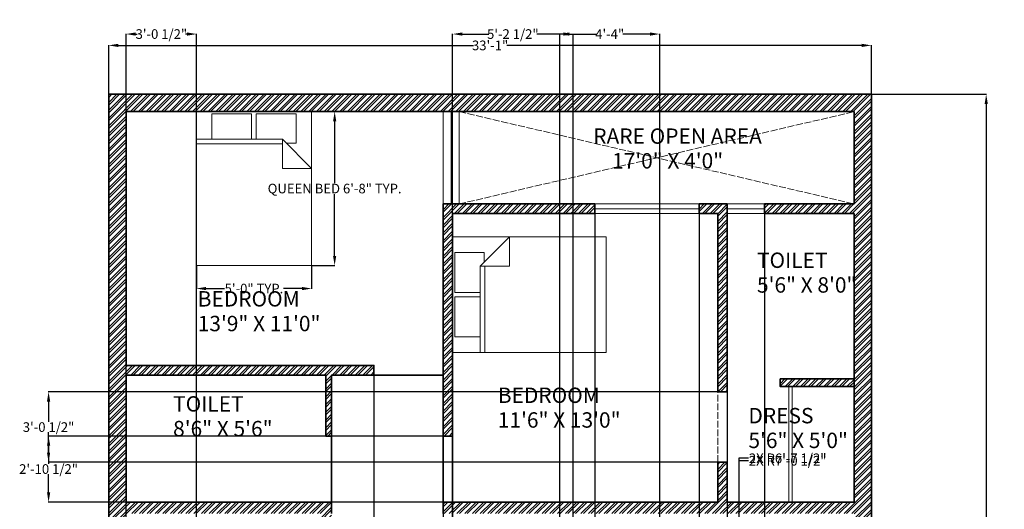
# Model space of a CAD drawing. Units: inches. Extents: x 334 to 846, y -424 to 250.
# Tile 3 of 3: x 334 to 846, y -5 to 250. Entities that reach past the tile are written whole.
import ezdxf

# ---------------------------------------------------------------- set-up
doc = ezdxf.new("R2010")
doc.units = ezdxf.units.IN
doc.header["$MEASUREMENT"] = 0
doc.linetypes.add('ACAD_ISO02W100', pattern=[15, 12, -3])
for name, color, linetype, lineweight in [('A-AREA-IDEN', 130, 'Continuous', 18), ('A-FLOR-FIXT', 8, 'Continuous', 18), ('A-FLOR-OPEN', 8, 'ACAD_ISO02W100', 13), ('A-WALL', 7, 'Continuous', 35), ('A-WALL-OVHD', 8, 'ACAD_ISO02W100', 18), ('A-WALL-PATT', 252, 'Continuous', 13), ('dimension', 130, 'Continuous', 18), ('furniture', 6, 'Continuous', 18), ('window', 150, 'Continuous', 18)]:
    doc.layers.add(name, color=color, linetype=linetype, lineweight=lineweight)
doc.styles.get("Standard").update_dxf_attribs({"font": 'arial.ttf'})
doc.dimstyles.get("Standard").update_dxf_attribs({"dimtxt": 5, "dimasz": 5, "dimexe": 0.18, "dimexo": 0.0625, "dimgap": 0.09, "dimtad": 0, "dimtih": 1, "dimtoh": 1, "dimdec": 1, "dimzin": 0, "dimdsep": 46, "dimlunit": 4, "dimtxsty": 'Standard', "dimcen": 0.09, "dimadec": 0, "dimazin": 0, "dimtfac": 1, "dimtdec": 1, "dimtofl": 0, "dimtmove": 0, "dimatfit": 3, "dimfxl": 1, "dimtolj": 1, "dimtzin": 0, "dimarcsym": 0})

# ---------------------------------------------------------------- blocks, each defined once
blk = doc.blocks.new('Bed - Queen')
for p, q in [((0, -80.00003), (0, 0)), ((0, 0), (59.99999, 0)), ((59.99999, 0), (59.99999, -80.00003)), ((7.99999, -1.2), (28.79998, -1.2)), ((7.99999, -14.4), (7.99999, -1.2)), ((28.79998, -1.2), (28.79998, -14.4)), ((31.19999, -1.2), (51.99999, -1.2)), ((31.19999, -14.4), (31.19999, -1.2)), ((51.99999, -1.2), (51.99999, -16.4)), ((0, -14.4), (44.8, -14.4)), ((59.99999, -29.6), (44.8, -14.4)), ((44.8, -14.4), (44.8, -29.6)), ((44.8, -16.8), (0, -16.8)), ((51.99999, -16.4), (46.79936, -16.4)), ((44.8, -29.6), (59.99999, -29.6)), ((59.99999, -80.00003), (0, -80.00003))]:
    blk.add_line(p, q)
blk = doc.blocks.new('*D7')
at = {"layer": 'Defpoints', "color": 0, "ltscale": 0.3, "transparency": 16777216}
for p in [(777.06, 236.45), (380.06, 211), (777.06, 211)]:
    blk.add_point(p, dxfattribs=at)
at = {"layer": 'dimension', "color": 0, "lineweight": -2, "ltscale": 0.3, "transparency": 16777216}
for p, q in [((380.06, 211.06), (380.06, 236.63)), ((385.06, 236.45), (569.89, 236.45)), ((772.06, 236.45), (587.24, 236.45)), ((777.06, 211.06), (777.06, 236.63))]:
    blk.add_line(p, q, dxfattribs=at)
at = {"layer": 'dimension', "color": 0, "ltscale": 0.3, "transparency": 16777216}
for points in [[(385.06, 237.28), (385.06, 235.61), (380.06, 236.45)], [(772.06, 237.28), (772.06, 235.61), (777.06, 236.45)]]:
    blk.add_solid(points, dxfattribs=at)
at = {"layer": 'dimension', "color": 0, "ltscale": 0.3, "transparency": 16777216, "insert": (578.56, 236.45), "char_height": 5, "attachment_point": 5}
blk.add_mtext('\\A1;33\'-1"', dxfattribs=at)
blk = doc.blocks.new('*D8')
at = {"layer": 'Defpoints', "color": 0, "ltscale": 0.3, "transparency": 16777216}
for p in [(777.06, 211), (777.06, -385), (836.82, -385)]:
    blk.add_point(p, dxfattribs=at)
at = {"layer": 'dimension', "color": 0, "lineweight": -2, "ltscale": 0.3, "transparency": 16777216}
for p, q in [((777.12, 211), (837, 211)), ((836.82, 206), (836.82, -84.36)), ((836.82, -380), (836.82, -89.65)), ((777.12, -385), (837, -385))]:
    blk.add_line(p, q, dxfattribs=at)
at = {"layer": 'dimension', "color": 0, "ltscale": 0.3, "transparency": 16777216}
for points in [[(835.99, 206), (837.66, 206), (836.82, 211)], [(835.99, -380), (837.66, -380), (836.82, -385)]]:
    blk.add_solid(points, dxfattribs=at)
at = {"layer": 'dimension', "color": 0, "ltscale": 0.3, "transparency": 16777216, "insert": (836.82, -87), "char_height": 5, "attachment_point": 5}
blk.add_mtext('\\A1;49\'-8"', dxfattribs=at)
blk = doc.blocks.new('*D10')
at = {"layer": 'Defpoints', "color": 0, "ltscale": 0.3, "transparency": 16777216}
for p in [(485.63, 202), (497.63, 202), (485.63, 122)]:
    blk.add_point(p, dxfattribs=at)
at = {"layer": 'dimension', "color": 0, "lineweight": -2, "ltscale": 0.3, "transparency": 16777216}
for p, q in [((485.69, 202), (497.81, 202)), ((497.63, 197), (497.63, 164.82)), ((497.63, 127), (497.63, 159.17)), ((485.69, 122), (497.81, 122))]:
    blk.add_line(p, q, dxfattribs=at)
at = {"layer": 'dimension', "color": 0, "ltscale": 0.3, "transparency": 16777216}
for points in [[(496.8, 197), (498.47, 197), (497.63, 202)], [(496.8, 127), (498.47, 127), (497.63, 122)]]:
    blk.add_solid(points, dxfattribs=at)
at = {"layer": 'dimension', "color": 0, "ltscale": 0.3, "transparency": 16777216, "insert": (497.63, 162), "char_height": 5, "attachment_point": 5}
blk.add_mtext('\\A1;QUEEN BED 6\'-8" TYP.', dxfattribs=at)
blk = doc.blocks.new('*D11')
at = {"layer": 'Defpoints', "color": 0, "ltscale": 0.3, "transparency": 16777216}
for p in [(425.63, 122), (485.63, 122), (485.63, 110)]:
    blk.add_point(p, dxfattribs=at)
at = {"layer": 'dimension', "color": 0, "lineweight": -2, "ltscale": 0.3, "transparency": 16777216}
for p, q in [((425.63, 121.93), (425.63, 109.82)), ((485.63, 121.93), (485.63, 109.82)), ((430.63, 110), (440.3, 110)), ((480.63, 110), (470.96, 110))]:
    blk.add_line(p, q, dxfattribs=at)
at = {"layer": 'dimension', "color": 0, "ltscale": 0.3, "transparency": 16777216}
for points in [[(430.63, 110.83), (430.63, 109.16), (425.63, 110)], [(480.63, 110.83), (480.63, 109.16), (485.63, 110)]]:
    blk.add_solid(points, dxfattribs=at)
at = {"layer": 'dimension', "color": 0, "ltscale": 0.3, "transparency": 16777216, "insert": (455.63, 110), "char_height": 5, "attachment_point": 5}
blk.add_mtext('\\A1;5\'-0" TYP.', dxfattribs=at)
blk = doc.blocks.new('*D20')
at = {"layer": 'Defpoints', "color": 0, "ltscale": 0.3, "transparency": 16777216}
for p in [(559.06, 149), (633.1, 149), (633.1, -416.35)]:
    blk.add_point(p, dxfattribs=at)
at = {"layer": 'dimension', "color": 0, "lineweight": -2, "ltscale": 0.3, "transparency": 16777216}
for p, q in [((559.06, 148.93), (559.06, -416.53)), ((633.1, 148.93), (633.1, -416.53)), ((564.06, -416.35), (589.33, -416.35)), ((628.1, -416.35), (602.83, -416.35))]:
    blk.add_line(p, q, dxfattribs=at)
at = {"layer": 'dimension', "color": 0, "ltscale": 0.3, "transparency": 16777216}
for points in [[(564.06, -415.52), (564.06, -417.19), (559.06, -416.35)], [(628.1, -415.52), (628.1, -417.19), (633.1, -416.35)]]:
    blk.add_solid(points, dxfattribs=at)
at = {"layer": 'dimension', "color": 0, "ltscale": 0.3, "transparency": 16777216, "insert": (596.08, -416.35), "char_height": 5, "attachment_point": 5}
blk.add_mtext('\\A1;6\'-2"', dxfattribs=at)
blk = doc.blocks.new('*D21')
at = {"layer": 'Defpoints', "color": 0, "ltscale": 0.3, "transparency": 16777216}
for p in [(633.1, 149), (687.41, 149), (687.41, -416.35)]:
    blk.add_point(p, dxfattribs=at)
at = {"layer": 'dimension', "color": 0, "lineweight": -2, "ltscale": 0.3, "transparency": 16777216}
for p, q in [((633.1, 148.93), (633.1, -416.53)), ((687.41, 148.93), (687.41, -416.53)), ((638.1, -416.35), (647.59, -416.35)), ((682.41, -416.35), (672.92, -416.35))]:
    blk.add_line(p, q, dxfattribs=at)
at = {"layer": 'dimension', "color": 0, "ltscale": 0.3, "transparency": 16777216}
for points in [[(638.1, -415.52), (638.1, -417.19), (633.1, -416.35)], [(682.41, -415.52), (682.41, -417.19), (687.41, -416.35)]]:
    blk.add_solid(points, dxfattribs=at)
at = {"layer": 'dimension', "color": 0, "ltscale": 0.3, "transparency": 16777216, "insert": (660.26, -416.35), "char_height": 5, "attachment_point": 5}
blk.add_mtext('\\A1;4\'-6 1/2"', dxfattribs=at)
blk = doc.blocks.new('*D22')
at = {"layer": 'Defpoints', "color": 0, "ltscale": 0.3, "transparency": 16777216}
for p in [(702.06, 149), (721.47, 149), (721.47, -416.35)]:
    blk.add_point(p, dxfattribs=at)
at = {"layer": 'dimension', "color": 0, "lineweight": -2, "ltscale": 0.3, "transparency": 16777216}
for p, q in [((702.06, 148.93), (702.06, -416.53)), ((721.47, 148.93), (721.47, -416.53)), ((707.06, -416.35), (716.47, -416.35)), ((721.47, -416.35), (726.47, -416.35))]:
    blk.add_line(p, q, dxfattribs=at)
at = {"layer": 'dimension', "color": 0, "ltscale": 0.3, "transparency": 16777216}
for points in [[(707.06, -415.52), (707.06, -417.19), (702.06, -416.35)], [(716.47, -415.52), (716.47, -417.19), (721.47, -416.35)]]:
    blk.add_solid(points, dxfattribs=at)
at = {"layer": 'dimension', "color": 0, "ltscale": 0.3, "transparency": 16777216, "insert": (738.8, -416.35), "char_height": 5, "attachment_point": 5}
blk.add_mtext('\\A1;1\'-7 1/2"', dxfattribs=at)
blk = doc.blocks.new('*D23')
at = {"layer": 'Defpoints', "color": 0, "ltscale": 0.3, "transparency": 16777216}
for p in [(518.06, 70), (554.06, 65), (554.06, -416.35)]:
    blk.add_point(p, dxfattribs=at)
at = {"layer": 'dimension', "color": 0, "lineweight": -2, "ltscale": 0.3, "transparency": 16777216}
for p, q in [((518.06, 69.93), (518.06, -416.53)), ((554.06, 64.93), (554.06, -416.53)), ((523.06, -416.35), (529.33, -416.35)), ((549.06, -416.35), (542.8, -416.35))]:
    blk.add_line(p, q, dxfattribs=at)
at = {"layer": 'dimension', "color": 0, "ltscale": 0.3, "transparency": 16777216}
for points in [[(523.06, -415.52), (523.06, -417.19), (518.06, -416.35)], [(549.06, -415.52), (549.06, -417.19), (554.06, -416.35)]]:
    blk.add_solid(points, dxfattribs=at)
at = {"layer": 'dimension', "color": 0, "ltscale": 0.3, "transparency": 16777216, "insert": (536.06, -416.35), "char_height": 5, "attachment_point": 5}
blk.add_mtext('\\A1;3\'-0"', dxfattribs=at)
blk = doc.blocks.new('*D24')
at = {"layer": 'Defpoints', "color": 0, "ltscale": 0.3, "transparency": 16777216}
for p in [(554.06, 33.31), (348.71, -1), (554.06, -1)]:
    blk.add_point(p, dxfattribs=at)
at = {"layer": 'dimension', "color": 0, "lineweight": -2, "ltscale": 0.3, "transparency": 16777216}
for p, q in [((554, 33.31), (348.53, 33.31)), ((348.71, 28.31), (348.71, 18.83)), ((348.71, 4), (348.71, 13.48)), ((554, -1), (348.53, -1))]:
    blk.add_line(p, q, dxfattribs=at)
at = {"layer": 'dimension', "color": 0, "ltscale": 0.3, "transparency": 16777216}
for points in [[(347.88, 28.31), (349.55, 28.31), (348.71, 33.31)], [(347.88, 4), (349.55, 4), (348.71, -1)]]:
    blk.add_solid(points, dxfattribs=at)
at = {"layer": 'dimension', "color": 0, "ltscale": 0.3, "transparency": 16777216, "insert": (348.71, 16.15), "char_height": 5, "attachment_point": 5}
blk.add_mtext('\\A1;2\'-10 1/2"', dxfattribs=at)
blk = doc.blocks.new('*D25')
at = {"layer": 'Defpoints', "color": 0, "ltscale": 0.3, "transparency": 16777216}
for p in [(496.06, 33.31), (348.71, -1), (496.06, -1)]:
    blk.add_point(p, dxfattribs=at)
at = {"layer": 'dimension', "color": 0, "lineweight": -2, "ltscale": 0.3, "transparency": 16777216}
for p, q in [((496, 33.31), (348.53, 33.31)), ((348.71, 28.31), (348.71, 18.83)), ((348.71, 4), (348.71, 13.48)), ((496, -1), (348.53, -1))]:
    blk.add_line(p, q, dxfattribs=at)
at = {"layer": 'dimension', "color": 0, "ltscale": 0.3, "transparency": 16777216}
for points in [[(347.88, 28.31), (349.55, 28.31), (348.71, 33.31)], [(347.88, 4), (349.55, 4), (348.71, -1)]]:
    blk.add_solid(points, dxfattribs=at)
at = {"layer": 'dimension', "color": 0, "ltscale": 0.3, "transparency": 16777216, "insert": (348.71, 16.15), "char_height": 5, "attachment_point": 5}
blk.add_mtext('\\A1;2\'-10 1/2"', dxfattribs=at)
blk = doc.blocks.new('*D26')
at = {"layer": 'Defpoints', "color": 0, "ltscale": 0.3, "transparency": 16777216}
for p in [(697.06, 56.25), (348.71, 19.69), (697.06, 19.69)]:
    blk.add_point(p, dxfattribs=at)
at = {"layer": 'dimension', "color": 0, "lineweight": -2, "ltscale": 0.3, "transparency": 16777216}
for p, q in [((697, 56.25), (348.53, 56.25)), ((348.71, 51.25), (348.71, 40.65)), ((348.71, 24.69), (348.71, 35.3)), ((697, 19.69), (348.53, 19.69))]:
    blk.add_line(p, q, dxfattribs=at)
at = {"layer": 'dimension', "color": 0, "ltscale": 0.3, "transparency": 16777216}
for points in [[(347.88, 51.25), (349.55, 51.25), (348.71, 56.25)], [(347.88, 24.69), (349.55, 24.69), (348.71, 19.69)]]:
    blk.add_solid(points, dxfattribs=at)
at = {"layer": 'dimension', "color": 0, "ltscale": 0.3, "transparency": 16777216, "insert": (348.71, 37.97), "char_height": 5, "attachment_point": 5}
blk.add_mtext('\\A1;3\'-0 1/2"', dxfattribs=at)
blk = doc.blocks.new('*D28')
at = {"layer": 'Defpoints', "color": 0, "ltscale": 0.3, "transparency": 16777216}
for p in [(666.86, 242.35), (614.79, -145), (666.86, -145)]:
    blk.add_point(p, dxfattribs=at)
at = {"layer": 'dimension', "color": 0, "lineweight": -2, "ltscale": 0.3, "transparency": 16777216}
for p, q in [((614.79, -144.94), (614.79, 242.53)), ((619.79, 242.35), (633.99, 242.35)), ((661.86, 242.35), (647.66, 242.35)), ((666.86, -144.94), (666.86, 242.53))]:
    blk.add_line(p, q, dxfattribs=at)
at = {"layer": 'dimension', "color": 0, "ltscale": 0.3, "transparency": 16777216}
for points in [[(619.79, 243.18), (619.79, 241.51), (614.79, 242.35)], [(661.86, 243.18), (661.86, 241.51), (666.86, 242.35)]]:
    blk.add_solid(points, dxfattribs=at)
at = {"layer": 'dimension', "color": 0, "ltscale": 0.3, "transparency": 16777216, "insert": (640.83, 242.35), "char_height": 5, "attachment_point": 5}
blk.add_mtext('\\A1;4\'-4"', dxfattribs=at)
blk = doc.blocks.new('*D30')
at = {"layer": 'Defpoints', "color": 0, "ltscale": 0.3, "transparency": 16777216}
for p in [(621.73, 242.35), (559.06, -271), (621.73, -271)]:
    blk.add_point(p, dxfattribs=at)
at = {"layer": 'dimension', "color": 0, "lineweight": -2, "ltscale": 0.3, "transparency": 16777216}
for p, q in [((559.06, -270.94), (559.06, 242.53)), ((564.06, 242.35), (577.83, 242.35)), ((616.73, 242.35), (602.96, 242.35)), ((621.73, -270.94), (621.73, 242.53))]:
    blk.add_line(p, q, dxfattribs=at)
at = {"layer": 'dimension', "color": 0, "ltscale": 0.3, "transparency": 16777216}
for points in [[(564.06, 243.18), (564.06, 241.51), (559.06, 242.35)], [(616.73, 243.18), (616.73, 241.51), (621.73, 242.35)]]:
    blk.add_solid(points, dxfattribs=at)
at = {"layer": 'dimension', "color": 0, "ltscale": 0.3, "transparency": 16777216, "insert": (590.4, 242.35), "char_height": 5, "attachment_point": 5}
blk.add_mtext('\\A1;5\'-2 1/2"', dxfattribs=at)
blk = doc.blocks.new('*D31')
at = {"layer": 'Defpoints', "color": 0, "ltscale": 0.3, "transparency": 16777216}
for p in [(425.8, 242.35), (389.06, -35.92), (425.8, -41.92)]:
    blk.add_point(p, dxfattribs=at)
at = {"layer": 'dimension', "color": 0, "lineweight": -2, "ltscale": 0.3, "transparency": 16777216}
for p, q in [((389.06, -35.86), (389.06, 242.53)), ((394.06, 242.35), (394.87, 242.35)), ((420.8, 242.35), (419.99, 242.35)), ((425.8, -41.86), (425.8, 242.53))]:
    blk.add_line(p, q, dxfattribs=at)
at = {"layer": 'dimension', "color": 0, "ltscale": 0.3, "transparency": 16777216}
for points in [[(394.06, 243.18), (394.06, 241.51), (389.06, 242.35)], [(420.8, 243.18), (420.8, 241.51), (425.8, 242.35)]]:
    blk.add_solid(points, dxfattribs=at)
at = {"layer": 'dimension', "color": 0, "ltscale": 0.3, "transparency": 16777216, "insert": (407.43, 242.35), "char_height": 5, "attachment_point": 5}
blk.add_mtext('\\A1;3\'-0 1/2"', dxfattribs=at)
blk = doc.blocks.new('*D34')
at = {"layer": 'Defpoints', "color": 0, "ltscale": 0.3, "transparency": 16777216}
for p in [(708.1, -30.1), (708.1, -114.35)]:
    blk.add_point(p, dxfattribs=at)
at = {"layer": 'dimension', "color": 0, "lineweight": -2, "ltscale": 0.3, "transparency": 16777216}
for p, q in [((713.1, 20.45), (708.1, 20.45)), ((708.1, 20.45), (708.1, -25.1)), ((708.01, -114.35), (708.19, -114.35)), ((708.1, -114.44), (708.1, -114.26))]:
    blk.add_line(p, q, dxfattribs=at)
at = {"layer": 'dimension', "color": 0, "ltscale": 0.3, "transparency": 16777216}
blk.add_solid([(707.27, -25.1), (708.93, -25.1), (708.1, -30.1)], dxfattribs=at)
at = {"layer": 'dimension', "color": 0, "ltscale": 0.3, "transparency": 16777216, "insert": (733.47, 20.45), "char_height": 5, "attachment_point": 5}
blk.add_mtext('\\A1;2X R7\'-0 1/2"', dxfattribs=at)
blk = doc.blocks.new('*D35')
at = {"layer": 'Defpoints', "color": 0, "ltscale": 0.3, "transparency": 16777216}
for p in [(708.1, -25.93), (708.1, -105.35)]:
    blk.add_point(p, dxfattribs=at)
at = {"layer": 'dimension', "color": 0, "lineweight": -2, "ltscale": 0.3, "transparency": 16777216}
for p, q in [((713.1, 21.73), (708.1, 21.73)), ((708.1, 21.73), (708.1, -20.93)), ((708.01, -105.35), (708.19, -105.35)), ((708.1, -105.44), (708.1, -105.26))]:
    blk.add_line(p, q, dxfattribs=at)
at = {"layer": 'dimension', "color": 0, "ltscale": 0.3, "transparency": 16777216}
blk.add_solid([(707.27, -20.93), (708.93, -20.93), (708.1, -25.93)], dxfattribs=at)
at = {"layer": 'dimension', "color": 0, "ltscale": 0.3, "transparency": 16777216, "insert": (733.47, 21.73), "char_height": 5, "attachment_point": 5}
blk.add_mtext('\\A1;2X R6\'-7 1/2"', dxfattribs=at)

msp = doc.modelspace()

# ---------------------------------------------------------------- hatches: boundary and pattern name
at = {"layer": 'A-WALL-PATT', "ltscale": 0.3}
h = msp.add_hatch(dxfattribs=at)
h.set_pattern_fill('ANSI32', color=256, scale=7.6)
h.paths.add_polyline_path([(559.06, 149), (633.1, 149), (633.1, 154), (559.06, 154), (554.06, 154), (554.06, 33.31), (559.06, 33.31)], flags=17)
h.paths.add_polyline_path([(777.06, 211), (380.06, 211), (380.06, -385), (389.06, -385), (389.06, -7), (490.06, -7), (490.06, -108.26), (496.06, -108.26), (496.06, -7), (496.06, -1), (389.06, -1), (389.06, 65), (493.06, 65), (493.06, 33.31), (496.06, 33.31), (496.06, 65), (518.06, 65), (518.06, 70), (389.06, 70), (389.06, 202), (554.06, 202), (562.49, 202), (768.06, 202), (768.06, 154), (721.47, 154), (721.47, 149), (768.06, 149), (768.06, -1), (702.06, -1), (702.06, 19.69), (697.06, 19.69), (697.06, -1), (554.06, -1), (554.06, -7), (697.06, -7), (768.06, -7), (768.06, -145), (702.06, -145), (697.06, -145), (666.86, -145), (666.86, -151), (697.06, -151), (702.06, -151), (768.06, -151), (768.06, -205), (735.06, -205), (735.06, -211), (768.06, -211), (768.06, -271), (758.48, -271), (758.48, -275), (768.06, -275), (768.06, -349), (768.06, -379), (702.06, -379), (697.06, -379), (559.06, -379), (559.06, -349), (559.06, -275), (566.23, -275), (566.23, -271), (559.06, -271), (559.06, -145), (554.06, -145), (554.06, -349), (554.06, -385), (559.06, -385), (697.06, -385), (702.06, -385), (768.06, -385), (777.06, -385), (777.06, -349)])
h = msp.add_hatch(dxfattribs=at)
h.set_pattern_fill('ANSI32', color=256, scale=7.6)
h.paths.add_polyline_path([(702.06, 154), (687.41, 154), (687.41, 149), (697.06, 149), (697.06, 56.25), (702.06, 56.25)], flags=17)
h.paths.add_polyline_path([(442.56, -139), (413.06, -139), (413.06, -145), (442.56, -145)], flags=17)
h.paths.add_polyline_path([(496.06, -139), (482.97, -139), (482.97, -145), (496.06, -145)], flags=17)
h.paths.add_polyline_path([(702.98, -271), (668.71, -271), (642.67, -271), (621.73, -271), (621.73, -275), (642.67, -275), (679.56, -275), (702.98, -275)], flags=17)
h.paths.add_polyline_path([(768.06, 63), (729.58, 63), (729.58, 59), (747.32, 59), (768.06, 59)], flags=17)

# ---------------------------------------------------------------- linework, layer by layer
at = {"layer": 'A-FLOR-FIXT', "ltscale": 0.3}
for p, q in [((734.16, 59), (734.16, -1)), ((735.74, 59), (735.74, -1))]:
    msp.add_line(p, q, dxfattribs=at)
at = {"layer": 'A-FLOR-OPEN', "ltscale": 0.3}
for p, q in [((562.49, 202), (768.06, 154)), ((562.49, 154), (768.06, 202))]:
    msp.add_line(p, q, dxfattribs=at)
at = {"layer": 'A-WALL', "ltscale": 0.3}
for p, q in [((554.06, 202), (559.06, 202)), ((559.06, 154), (554.06, 154)), ((633.1, 154), (633.1, 149)), ((687.41, 154), (687.41, 149)), ((721.47, 154), (721.47, 149)), ((697.06, 56.25), (702.06, 56.25)), ((554.06, 33.31), (559.06, 33.31)), ((697.06, 19.69), (702.06, 19.69))]:
    msp.add_line(p, q, dxfattribs=at)
at = {"layer": 'A-WALL'}
for p, q in [((559.06, 202), (768.06, 202)), ((768.06, 202), (768.06, 154)), ((554.06, 154), (554.06, -7)), ((559.06, 154), (633.1, 154)), ((687.41, 154), (702.06, 154)), ((702.06, 154), (702.06, 56.25)), ((721.47, 154), (768.06, 154)), ((559.06, 149), (633.1, 149)), ((559.06, 149), (559.06, 33.31)), ((687.41, 149), (697.06, 149)), ((697.06, 149), (697.06, 56.25)), ((721.47, 149), (768.06, 149)), ((768.06, 149), (768.06, -1)), ((697.06, 19.69), (697.06, -1)), ((702.06, 19.69), (702.06, -1)), ((496.06, -1), (496.06, -7)), ((554.06, -1), (697.06, -1)), ((702.06, -1), (768.06, -1))]:
    msp.add_line(p, q, dxfattribs=at)
at = {"layer": 'A-WALL', "ltscale": 0.3}
for points in [[(554.06, -385), (559.06, -385), (697.06, -385), (702.06, -385), (768.06, -385), (777.06, -385), (777.06, -349), (777.06, 211), (380.06, 211), (380.06, -385)], [(768.06, 59), (747.32, 59), (729.58, 59), (729.58, 63), (768.06, 63)]]:
    msp.add_lwpolyline(points, dxfattribs=at)
at = {"layer": 'A-WALL'}
for points in [[(554.06, 202), (389.06, 202), (389.06, 70), (518.06, 70), (518.06, 65)], [(496.06, -1), (389.06, -1), (389.06, 65), (493.06, 65), (493.06, 33.31), (496.06, 33.31)], [(496.06, -2.56), (496.06, 65), (554.06, 65)]]:
    msp.add_lwpolyline(points, dxfattribs=at)
at = {"layer": 'A-WALL-OVHD', "ltscale": 0.3}
msp.add_line((496.06, -1), (554.06, -1), dxfattribs=at)
msp.add_lwpolyline([(697.06, 56.25), (702.06, 56.25), (702.06, 19.69), (697.06, 19.69)], close=True, dxfattribs=at)
at = {"layer": 'window', "ltscale": 0.3}
for p, q in [((558.28, 202), (558.28, 154)), ((633.1, 151.5), (687.41, 151.5)), ((702.06, 151.5), (721.47, 151.5))]:
    msp.add_line(p, q, dxfattribs=at)
for points in [[(554.06, 202), (562.49, 202), (562.49, 154), (554.06, 154)], [(633.1, 154), (687.41, 154), (687.41, 149), (633.1, 149)], [(721.47, 154), (702.06, 154), (702.06, 149), (721.47, 149)]]:
    msp.add_lwpolyline(points, close=True, dxfattribs=at)

# ---------------------------------------------------------------- block references
at = {"layer": 'furniture', "ltscale": 0.3}
msp.add_blockref('Bed - Queen', (425.63, 202), dxfattribs=at)
at = {"layer": 'furniture', "ltscale": 0.3, "rotation": 90}
msp.add_blockref('Bed - Queen', (559.06, 76.82), dxfattribs=at)

# ---------------------------------------------------------------- texts
at = {"layer": 'A-AREA-IDEN', "ltscale": 0.3}
for s, p in [('RARE OPEN AREA', (632.26, 185.27)), ('    17\'0" X 4\'0"', (632.26, 172.42)), ('TOILET', (717.49, 120.73)), ('5\'6" X 8\'0"', (717.49, 107.88)), ('BEDROOM', (426.34, 100.66)), ('13\'9" X 11\'0"', (426.34, 87.81)), ('BEDROOM ', (582.57, 50.51)), ('TOILET', (413.53, 46.03)), ('DRESS', (713.03, 39.91)), ('8\'6" X 5\'6"', (413.53, 33.18)), ('11\'6" X 13\'0"', (582.57, 37.66)), ('5\'6" X 5\'0"', (713.03, 27.05))]:
    msp.add_text(s, height=8, dxfattribs=at).set_placement(p)

# ---------------------------------------------------------------- dimensions: what is measured, and where the dimension line sits
at = {"layer": 'dimension', "ltscale": 0.3}
for base, p1, p2, override, picture, middle in [((425.8, 242.35), (389.06, -35.92), (425.8, -41.92), {"dimdec": 1, "dimlfac": 1, "dimrnd": 0, "dimzin": 1, "dimdsep": 46, "dimlunit": 4, "dimfrac": 2}, '*D31', (407.43, 242.35)), ((621.73, 242.35), (559.06, -271), (621.73, -271), {"dimdec": 1, "dimlfac": 1, "dimrnd": 0, "dimzin": 1, "dimdsep": 46, "dimlunit": 4, "dimfrac": 2}, '*D30', (590.4, 242.35)), ((666.86, 242.35), (614.79, -145), (666.86, -145), {"dimdec": 1, "dimlfac": 1, "dimrnd": 0, "dimzin": 1, "dimdsep": 46, "dimlunit": 4, "dimfrac": 2}, '*D28', (640.83, 242.35)), ((777.06, 236.45), (380.06, 211), (777.06, 211), {"dimclrd": 0, "dimclre": 0, "dimclrt": 0}, '*D7', (578.56, 236.45)), ((633.1, -416.35), (559.06, 149), (633.1, 149), {"dimdec": 1, "dimlfac": 1, "dimrnd": 0, "dimzin": 1, "dimdsep": 46, "dimlunit": 4, "dimfrac": 2}, '*D20', (596.08, -416.35)), ((687.41, -416.35), (633.1, 149), (687.41, 149), {"dimdec": 1, "dimlfac": 1, "dimrnd": 0, "dimzin": 1, "dimdsep": 46, "dimlunit": 4, "dimfrac": 2}, '*D21', (660.26, -416.35)), ((721.47, -416.35), (702.06, 149), (721.47, 149), {"dimdec": 1, "dimlfac": 1, "dimrnd": 0, "dimzin": 1, "dimdsep": 46, "dimlunit": 4, "dimfrac": 2}, '*D22', (738.8, -416.35)), ((554.06, -416.35), (518.06, 70), (554.06, 65), {"dimdec": 1, "dimlfac": 1, "dimrnd": 0, "dimzin": 1, "dimdsep": 46, "dimlunit": 4, "dimfrac": 2}, '*D23', (536.06, -416.35))]:
    dim = msp.add_linear_dim(base=base, p1=p1, p2=p2, dimstyle='Standard', override=override, dxfattribs=at)
    dim.commit()
    dim.dimension.update_dxf_attribs({"geometry": picture, "text_midpoint": middle})
for base, p1, p2, override, picture, middle in [((836.82, -385), (777.06, 211), (777.06, -385), {"dimclrd": 0, "dimclre": 0, "dimclrt": 0}, '*D8', (836.82, -87)), ((348.71, 19.69), (697.06, 56.25), (697.06, 19.69), {"dimdec": 1, "dimlfac": 1, "dimrnd": 0, "dimzin": 1, "dimdsep": 46, "dimlunit": 4, "dimfrac": 2}, '*D26', (348.71, 37.97)), ((348.71, -1), (554.06, 33.31), (554.06, -1), {"dimdec": 1, "dimlfac": 1, "dimrnd": 0, "dimzin": 1, "dimdsep": 46, "dimlunit": 4, "dimfrac": 2}, '*D24', (348.71, 16.15)), ((348.71, -1), (496.06, 33.31), (496.06, -1), {"dimdec": 1, "dimlfac": 1, "dimrnd": 0, "dimzin": 1, "dimdsep": 46, "dimlunit": 4, "dimfrac": 2}, '*D25', (348.71, 16.15))]:
    dim = msp.add_linear_dim(base=base, p1=p1, p2=p2, angle=90, dimstyle='Standard', override=override, dxfattribs=at)
    dim.commit()
    dim.dimension.update_dxf_attribs({"geometry": picture, "text_midpoint": middle})
dim = msp.add_linear_dim(base=(497.63, 202), p1=(485.63, 122), p2=(485.63, 202), angle=90, text='QUEEN BED <> TYP.', dimstyle='Standard', override={"dimdec": 1, "dimlfac": 1, "dimrnd": 0, "dimzin": 1, "dimdsep": 46, "dimlunit": 4, "dimfrac": 2}, dxfattribs=at)
dim.commit()
dim.dimension.update_dxf_attribs({"geometry": '*D10', "text_midpoint": (497.63, 162)})
dim = msp.add_linear_dim(base=(485.63, 110), p1=(425.63, 122), p2=(485.63, 122), text='<> TYP.', dimstyle='Standard', override={"dimdec": 1, "dimlfac": 1, "dimrnd": 0, "dimzin": 1, "dimdsep": 46, "dimlunit": 4, "dimfrac": 2}, dxfattribs=at)
dim.commit()
dim.dimension.update_dxf_attribs({"geometry": '*D11', "text_midpoint": (455.63, 110)})
for center, mpoint, picture, middle in [((708.1, -105.35), (708.1, -25.93), '*D35', (733.47, 21.73)), ((708.0998, -114.3517), (708.1, -30.0975), '*D34', (733.4681, 20.455))]:
    dim = msp.add_radius_dim(center=center, mpoint=mpoint, text='2X <>', dimstyle='Standard', override={"dimdec": 1, "dimlfac": 1, "dimrnd": 0, "dimzin": 1, "dimdsep": 46, "dimlunit": 4, "dimfrac": 2}, dxfattribs=at)
    dim.commit()
    dim.dimension.update_dxf_attribs({"geometry": picture, "text_midpoint": middle, "dimtype": 164})

doc.saveas('drawing.dxf')
